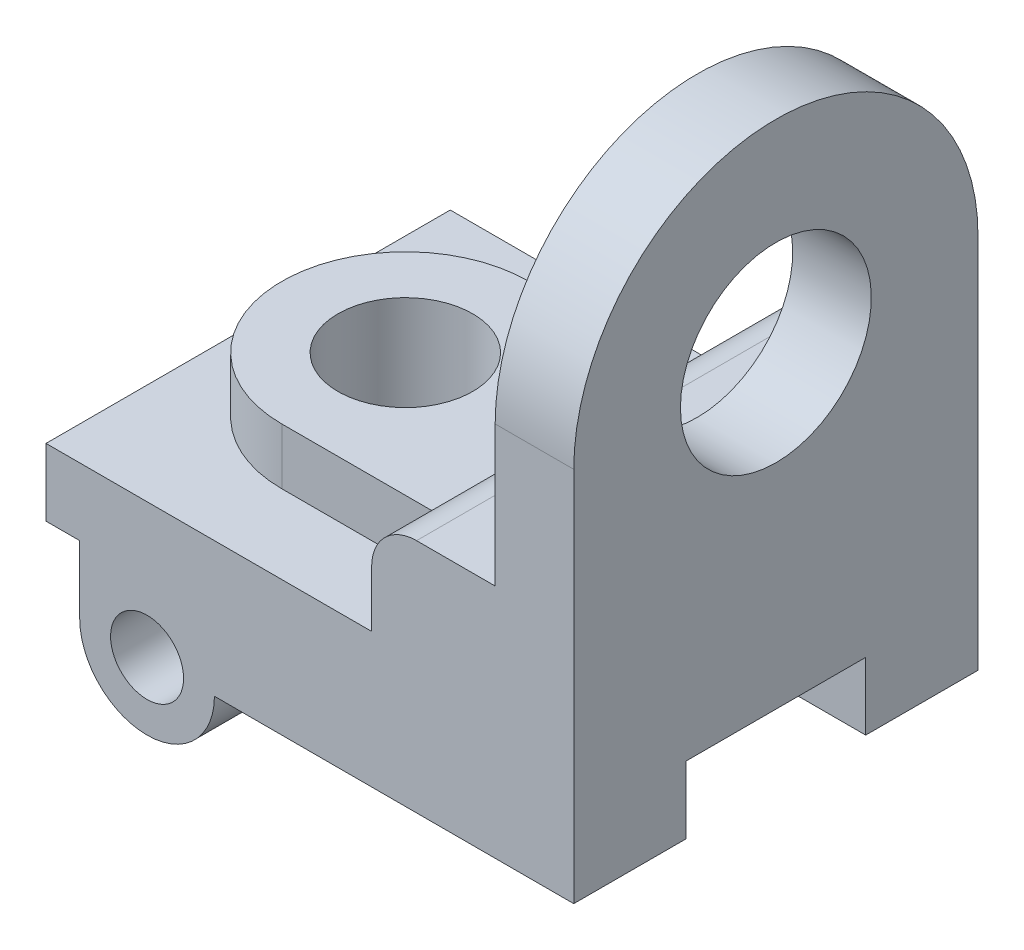
ISO-10303-21;
HEADER;
FILE_DESCRIPTION(('STEP AP214'),'2;1');
FILE_NAME('part.step','',(''),(''),'','','');
FILE_SCHEMA(('AUTOMOTIVE_DESIGN { 1 0 10303 214 1 1 1 1 }'));
ENDSEC;
DATA;
#1=APPLICATION_CONTEXT('core data for automotive mechanical design processes');
#2=APPLICATION_PROTOCOL_DEFINITION('international standard','automotive_design',2000,#1);
#3=PRODUCT_CONTEXT('',#1,'mechanical');
#4=PRODUCT('Part','Part','',(#3));
#5=PRODUCT_RELATED_PRODUCT_CATEGORY('part','',(#4));
#6=PRODUCT_DEFINITION_FORMATION('','',#4);
#7=PRODUCT_DEFINITION_CONTEXT('part definition',#1,'design');
#8=PRODUCT_DEFINITION('design','',#6,#7);
#9=PRODUCT_DEFINITION_SHAPE('','',#8);
#10=(LENGTH_UNIT() NAMED_UNIT(*) SI_UNIT(.MILLI.,.METRE.));
#11=(NAMED_UNIT(*) PLANE_ANGLE_UNIT() SI_UNIT($,.RADIAN.));
#12=(NAMED_UNIT(*) SI_UNIT($,.STERADIAN.) SOLID_ANGLE_UNIT());
#13=UNCERTAINTY_MEASURE_WITH_UNIT(LENGTH_MEASURE(1.E-05),#10,'distance_accuracy_value','');
#14=(GEOMETRIC_REPRESENTATION_CONTEXT(3) GLOBAL_UNCERTAINTY_ASSIGNED_CONTEXT((#13)) GLOBAL_UNIT_ASSIGNED_CONTEXT((#10,
#11,#12)) REPRESENTATION_CONTEXT('',''));
#15=CARTESIAN_POINT('',(0.,0.,0.));
#16=DIRECTION('',(0.,0.,1.));
#17=DIRECTION('',(1.,0.,0.));
#18=AXIS2_PLACEMENT_3D('',#15,#16,#17);
#19=CARTESIAN_POINT('',(-36.,0.,36.));
#20=DIRECTION('',(1.,0.,0.));
#21=DIRECTION('',(0.,0.,-1.));
#22=AXIS2_PLACEMENT_3D('',#19,#20,#21);
#23=PLANE('',#22);
#24=DIRECTION('',(0.,-1.,0.));
#25=VECTOR('',#24,1.);
#26=CARTESIAN_POINT('',(-36.,22.,22.));
#27=LINE('',#26,#25);
#28=CARTESIAN_POINT('',(-36.,22.,22.));
#29=VERTEX_POINT('',#28);
#30=CARTESIAN_POINT('',(-36.,12.,22.));
#31=VERTEX_POINT('',#30);
#32=EDGE_CURVE('E198',#29,#31,#27,.T.);
#33=ORIENTED_EDGE('',*,*,#32,.T.);
#34=DIRECTION('',(0.,0.,-1.));
#35=VECTOR('',#34,1.);
#36=CARTESIAN_POINT('',(-36.,12.,36.));
#37=LINE('',#36,#35);
#38=CARTESIAN_POINT('',(-36.,12.,36.));
#39=VERTEX_POINT('',#38);
#40=EDGE_CURVE('E329',#39,#31,#37,.T.);
#41=ORIENTED_EDGE('',*,*,#40,.F.);
#42=DIRECTION('',(0.,-1.,0.));
#43=VECTOR('',#42,1.);
#44=CARTESIAN_POINT('',(-36.,0.,36.));
#45=LINE('',#44,#43);
#46=CARTESIAN_POINT('',(-36.,22.,36.));
#47=VERTEX_POINT('',#46);
#48=EDGE_CURVE('E276',#47,#39,#45,.T.);
#49=ORIENTED_EDGE('',*,*,#48,.F.);
#50=DIRECTION('',(0.,0.,-1.));
#51=VECTOR('',#50,1.);
#52=CARTESIAN_POINT('',(-36.,22.,36.));
#53=LINE('',#52,#51);
#54=EDGE_CURVE('E331',#47,#29,#53,.T.);
#55=ORIENTED_EDGE('',*,*,#54,.T.);
#56=EDGE_LOOP('',(#33,#41,#49,#55));
#57=FACE_BOUND('',#56,.T.);
#58=ADVANCED_FACE('F41',(#57),#23,.F.);
#59=DIRECTION('',(0.,-1.,0.));
#60=VECTOR('',#59,1.);
#61=CARTESIAN_POINT('',(-36.,22.,-22.));
#62=LINE('',#61,#60);
#63=CARTESIAN_POINT('',(-36.,22.,-22.));
#64=VERTEX_POINT('',#63);
#65=CARTESIAN_POINT('',(-36.,12.,-22.));
#66=VERTEX_POINT('',#65);
#67=EDGE_CURVE('E59',#64,#66,#62,.T.);
#68=ORIENTED_EDGE('',*,*,#67,.F.);
#69=CARTESIAN_POINT('',(-36.,22.,-36.));
#70=VERTEX_POINT('',#69);
#71=EDGE_CURVE('E334',#64,#70,#53,.T.);
#72=ORIENTED_EDGE('',*,*,#71,.T.);
#73=DIRECTION('',(0.,-1.,0.));
#74=VECTOR('',#73,1.);
#75=CARTESIAN_POINT('',(-36.,0.,-36.));
#76=LINE('',#75,#74);
#77=CARTESIAN_POINT('',(-36.,12.,-36.));
#78=VERTEX_POINT('',#77);
#79=EDGE_CURVE('E313',#70,#78,#76,.T.);
#80=ORIENTED_EDGE('',*,*,#79,.T.);
#81=EDGE_CURVE('E328',#66,#78,#37,.T.);
#82=ORIENTED_EDGE('',*,*,#81,.F.);
#83=EDGE_LOOP('',(#68,#72,#80,#82));
#84=FACE_BOUND('',#83,.T.);
#85=ADVANCED_FACE('F436',(#84),#23,.F.);
#86=CARTESIAN_POINT('',(0.,12.,36.));
#87=DIRECTION('',(0.,-1.,0.));
#88=DIRECTION('',(1.,0.,0.));
#89=AXIS2_PLACEMENT_3D('',#86,#87,#88);
#90=PLANE('',#89);
#91=DIRECTION('',(1.,0.,0.));
#92=VECTOR('',#91,1.);
#93=CARTESIAN_POINT('',(-66.,12.,22.));
#94=LINE('',#93,#92);
#95=CARTESIAN_POINT('',(-66.,12.,22.));
#96=VERTEX_POINT('',#95);
#97=EDGE_CURVE('E448',#96,#31,#94,.T.);
#98=ORIENTED_EDGE('',*,*,#97,.F.);
#99=CARTESIAN_POINT('',(-66.,12.,0.));
#100=DIRECTION('',(0.,1.,0.));
#101=DIRECTION('',(-1.,0.,0.));
#102=AXIS2_PLACEMENT_3D('',#99,#100,#101);
#103=CIRCLE('',#102,22.);
#104=CARTESIAN_POINT('',(-66.,12.,-22.));
#105=VERTEX_POINT('',#104);
#106=EDGE_CURVE('E209',#105,#96,#103,.T.);
#107=ORIENTED_EDGE('',*,*,#106,.F.);
#108=DIRECTION('',(-1.,0.,0.));
#109=VECTOR('',#108,1.);
#110=CARTESIAN_POINT('',(-66.,12.,-22.));
#111=LINE('',#110,#109);
#112=EDGE_CURVE('E210',#66,#105,#111,.T.);
#113=ORIENTED_EDGE('',*,*,#112,.F.);
#114=ORIENTED_EDGE('',*,*,#81,.T.);
#115=DIRECTION('',(-1.,0.,0.));
#116=VECTOR('',#115,1.);
#117=CARTESIAN_POINT('',(0.,12.,-36.));
#118=LINE('',#117,#116);
#119=CARTESIAN_POINT('',(-94.,12.,-36.));
#120=VERTEX_POINT('',#119);
#121=EDGE_CURVE('E314',#78,#120,#118,.T.);
#122=ORIENTED_EDGE('',*,*,#121,.T.);
#123=DIRECTION('',(0.,0.,-1.));
#124=VECTOR('',#123,1.);
#125=CARTESIAN_POINT('',(-94.,12.,36.));
#126=LINE('',#125,#124);
#127=CARTESIAN_POINT('',(-94.,12.,36.));
#128=VERTEX_POINT('',#127);
#129=EDGE_CURVE('E326',#128,#120,#126,.T.);
#130=ORIENTED_EDGE('',*,*,#129,.F.);
#131=DIRECTION('',(-1.,0.,0.));
#132=VECTOR('',#131,1.);
#133=CARTESIAN_POINT('',(0.,12.,36.));
#134=LINE('',#133,#132);
#135=EDGE_CURVE('E283',#39,#128,#134,.T.);
#136=ORIENTED_EDGE('',*,*,#135,.F.);
#137=ORIENTED_EDGE('',*,*,#40,.T.);
#138=EDGE_LOOP('',(#98,#107,#113,#114,#122,#130,#136,#137));
#139=FACE_BOUND('',#138,.T.);
#140=ADVANCED_FACE('F418',(#139),#90,.F.);
#141=CARTESIAN_POINT('',(-88.,0.,36.));
#142=DIRECTION('',(1.,0.,0.));
#143=DIRECTION('',(0.,0.,-1.));
#144=AXIS2_PLACEMENT_3D('',#141,#142,#143);
#145=PLANE('',#144);
#146=DIRECTION('',(0.,0.,-1.));
#147=VECTOR('',#146,1.);
#148=CARTESIAN_POINT('',(-88.,-12.,36.));
#149=LINE('',#148,#147);
#150=CARTESIAN_POINT('',(-88.,-12.,-16.));
#151=VERTEX_POINT('',#150);
#152=CARTESIAN_POINT('',(-88.,-12.,-36.));
#153=VERTEX_POINT('',#152);
#154=EDGE_CURVE('E49',#151,#153,#149,.T.);
#155=ORIENTED_EDGE('',*,*,#154,.F.);
#156=DIRECTION('',(0.,-1.,0.));
#157=VECTOR('',#156,1.);
#158=CARTESIAN_POINT('',(-88.,0.,-16.));
#159=LINE('',#158,#157);
#160=CARTESIAN_POINT('',(-88.,0.,-16.));
#161=VERTEX_POINT('',#160);
#162=EDGE_CURVE('E223',#161,#151,#159,.T.);
#163=ORIENTED_EDGE('',*,*,#162,.F.);
#164=DIRECTION('',(0.,0.,-1.));
#165=VECTOR('',#164,1.);
#166=CARTESIAN_POINT('',(-88.,0.,36.));
#167=LINE('',#166,#165);
#168=CARTESIAN_POINT('',(-88.,0.,-36.));
#169=VERTEX_POINT('',#168);
#170=EDGE_CURVE('E290',#161,#169,#167,.T.);
#171=ORIENTED_EDGE('',*,*,#170,.T.);
#172=DIRECTION('',(0.,-1.,0.));
#173=VECTOR('',#172,1.);
#174=CARTESIAN_POINT('',(-88.,0.,-36.));
#175=LINE('',#174,#173);
#176=EDGE_CURVE('E289',#169,#153,#175,.T.);
#177=ORIENTED_EDGE('',*,*,#176,.T.);
#178=EDGE_LOOP('',(#155,#163,#171,#177));
#179=FACE_BOUND('',#178,.T.);
#180=ADVANCED_FACE('F435',(#179),#145,.F.);
#181=CARTESIAN_POINT('',(-76.,-12.,36.));
#182=DIRECTION('',(0.,0.,-1.));
#183=DIRECTION('',(-1.,0.,0.));
#184=AXIS2_PLACEMENT_3D('',#181,#182,#183);
#185=CYLINDRICAL_SURFACE('',#184,12.);
#186=DIRECTION('',(0.,0.,-1.));
#187=VECTOR('',#186,1.);
#188=CARTESIAN_POINT('',(-64.,-12.,36.));
#189=LINE('',#188,#187);
#190=CARTESIAN_POINT('',(-64.,-12.,-16.));
#191=VERTEX_POINT('',#190);
#192=CARTESIAN_POINT('',(-64.,-12.,-36.));
#193=VERTEX_POINT('',#192);
#194=EDGE_CURVE('E347',#191,#193,#189,.T.);
#195=ORIENTED_EDGE('',*,*,#194,.F.);
#196=CARTESIAN_POINT('',(-76.,-12.,-16.));
#197=DIRECTION('',(0.,0.,-1.));
#198=DIRECTION('',(-1.,0.,0.));
#199=AXIS2_PLACEMENT_3D('',#196,#197,#198);
#200=CIRCLE('',#199,12.);
#201=EDGE_CURVE('E254',#191,#151,#200,.T.);
#202=ORIENTED_EDGE('',*,*,#201,.T.);
#203=ORIENTED_EDGE('',*,*,#154,.T.);
#204=CARTESIAN_POINT('',(-76.,-12.,-36.));
#205=DIRECTION('',(0.,0.,1.));
#206=DIRECTION('',(1.,0.,0.));
#207=AXIS2_PLACEMENT_3D('',#204,#205,#206);
#208=CIRCLE('',#207,12.);
#209=EDGE_CURVE('E291',#153,#193,#208,.T.);
#210=ORIENTED_EDGE('',*,*,#209,.T.);
#211=EDGE_LOOP('',(#195,#202,#203,#210));
#212=FACE_BOUND('',#211,.T.);
#213=ADVANCED_FACE('F495',(#212),#185,.T.);
#214=CARTESIAN_POINT('',(0.,-12.,36.));
#215=DIRECTION('',(0.,1.,0.));
#216=DIRECTION('',(0.,0.,1.));
#217=AXIS2_PLACEMENT_3D('',#214,#215,#216);
#218=PLANE('',#217);
#219=DIRECTION('',(0.,0.,-1.));
#220=VECTOR('',#219,1.);
#221=CARTESIAN_POINT('',(0.,-12.,36.));
#222=LINE('',#221,#220);
#223=CARTESIAN_POINT('',(0.,-12.,-16.));
#224=VERTEX_POINT('',#223);
#225=CARTESIAN_POINT('',(0.,-12.,-36.));
#226=VERTEX_POINT('',#225);
#227=EDGE_CURVE('E345',#224,#226,#222,.T.);
#228=ORIENTED_EDGE('',*,*,#227,.F.);
#229=DIRECTION('',(-1.,0.,0.));
#230=VECTOR('',#229,1.);
#231=CARTESIAN_POINT('',(0.,-12.,-16.));
#232=LINE('',#231,#230);
#233=EDGE_CURVE('E252',#224,#191,#232,.T.);
#234=ORIENTED_EDGE('',*,*,#233,.T.);
#235=ORIENTED_EDGE('',*,*,#194,.T.);
#236=DIRECTION('',(1.,0.,0.));
#237=VECTOR('',#236,1.);
#238=CARTESIAN_POINT('',(0.,-12.,-36.));
#239=LINE('',#238,#237);
#240=EDGE_CURVE('E298',#193,#226,#239,.T.);
#241=ORIENTED_EDGE('',*,*,#240,.T.);
#242=EDGE_LOOP('',(#228,#234,#235,#241));
#243=FACE_BOUND('',#242,.T.);
#244=ADVANCED_FACE('F426',(#243),#218,.F.);
#245=CARTESIAN_POINT('',(-76.,-12.,36.));
#246=DIRECTION('',(0.,0.,-1.));
#247=DIRECTION('',(-1.,0.,0.));
#248=AXIS2_PLACEMENT_3D('',#245,#246,#247);
#249=CYLINDRICAL_SURFACE('',#248,6.5);
#250=CARTESIAN_POINT('',(-76.,-12.,-16.));
#251=DIRECTION('',(0.,0.,-1.));
#252=DIRECTION('',(-1.,0.,0.));
#253=AXIS2_PLACEMENT_3D('',#250,#251,#252);
#254=CIRCLE('',#253,6.5);
#255=CARTESIAN_POINT('',(-82.5,-12.,-16.));
#256=VERTEX_POINT('',#255);
#257=EDGE_CURVE('E44',#256,#256,#254,.T.);
#258=ORIENTED_EDGE('',*,*,#257,.F.);
#259=EDGE_LOOP('',(#258));
#260=FACE_BOUND('',#259,.T.);
#261=CARTESIAN_POINT('',(-76.,-12.,-36.));
#262=DIRECTION('',(0.,0.,1.));
#263=DIRECTION('',(1.,0.,0.));
#264=AXIS2_PLACEMENT_3D('',#261,#262,#263);
#265=CIRCLE('',#264,6.5);
#266=CARTESIAN_POINT('',(-69.5,-12.,-36.));
#267=VERTEX_POINT('',#266);
#268=EDGE_CURVE('E260',#267,#267,#265,.T.);
#269=ORIENTED_EDGE('',*,*,#268,.F.);
#270=EDGE_LOOP('',(#269));
#271=FACE_BOUND('',#270,.T.);
#272=ADVANCED_FACE('F357',(#260,#271),#249,.F.);
#273=CARTESIAN_POINT('',(-88.,0.,36.));
#274=VERTEX_POINT('',#273);
#275=CARTESIAN_POINT('',(-88.,0.,16.));
#276=VERTEX_POINT('',#275);
#277=EDGE_CURVE('E319',#274,#276,#167,.T.);
#278=ORIENTED_EDGE('',*,*,#277,.T.);
#279=DIRECTION('',(0.,1.,0.));
#280=VECTOR('',#279,1.);
#281=CARTESIAN_POINT('',(-88.,0.,16.));
#282=LINE('',#281,#280);
#283=CARTESIAN_POINT('',(-88.,-12.,16.));
#284=VERTEX_POINT('',#283);
#285=EDGE_CURVE('E235',#284,#276,#282,.T.);
#286=ORIENTED_EDGE('',*,*,#285,.F.);
#287=CARTESIAN_POINT('',(-88.,-12.,36.));
#288=VERTEX_POINT('',#287);
#289=EDGE_CURVE('E11',#288,#284,#149,.T.);
#290=ORIENTED_EDGE('',*,*,#289,.F.);
#291=DIRECTION('',(0.,-1.,0.));
#292=VECTOR('',#291,1.);
#293=CARTESIAN_POINT('',(-88.,0.,36.));
#294=LINE('',#293,#292);
#295=EDGE_CURVE('E261',#274,#288,#294,.T.);
#296=ORIENTED_EDGE('',*,*,#295,.F.);
#297=EDGE_LOOP('',(#278,#286,#290,#296));
#298=FACE_BOUND('',#297,.T.);
#299=ADVANCED_FACE('F372',(#298),#145,.F.);
#300=CARTESIAN_POINT('',(-76.,-12.,16.));
#301=DIRECTION('',(0.,0.,1.));
#302=DIRECTION('',(0.,-1.,0.));
#303=AXIS2_PLACEMENT_3D('',#300,#301,#302);
#304=CIRCLE('',#303,12.);
#305=CARTESIAN_POINT('',(-64.,-12.,16.));
#306=VERTEX_POINT('',#305);
#307=EDGE_CURVE('E249',#284,#306,#304,.T.);
#308=ORIENTED_EDGE('',*,*,#307,.T.);
#309=CARTESIAN_POINT('',(-64.,-12.,36.));
#310=VERTEX_POINT('',#309);
#311=EDGE_CURVE('E350',#310,#306,#189,.T.);
#312=ORIENTED_EDGE('',*,*,#311,.F.);
#313=CARTESIAN_POINT('',(-76.,-12.,36.));
#314=DIRECTION('',(0.,0.,1.));
#315=DIRECTION('',(1.,0.,0.));
#316=AXIS2_PLACEMENT_3D('',#313,#314,#315);
#317=CIRCLE('',#316,12.);
#318=EDGE_CURVE('E264',#288,#310,#317,.T.);
#319=ORIENTED_EDGE('',*,*,#318,.F.);
#320=ORIENTED_EDGE('',*,*,#289,.T.);
#321=EDGE_LOOP('',(#308,#312,#319,#320));
#322=FACE_BOUND('',#321,.T.);
#323=ADVANCED_FACE('F376',(#322),#185,.T.);
#324=ORIENTED_EDGE('',*,*,#311,.T.);
#325=DIRECTION('',(1.,0.,0.));
#326=VECTOR('',#325,1.);
#327=CARTESIAN_POINT('',(0.,-12.,16.));
#328=LINE('',#327,#326);
#329=CARTESIAN_POINT('',(0.,-12.,16.));
#330=VERTEX_POINT('',#329);
#331=EDGE_CURVE('E250',#306,#330,#328,.T.);
#332=ORIENTED_EDGE('',*,*,#331,.T.);
#333=CARTESIAN_POINT('',(0.,-12.,36.));
#334=VERTEX_POINT('',#333);
#335=EDGE_CURVE('E343',#334,#330,#222,.T.);
#336=ORIENTED_EDGE('',*,*,#335,.F.);
#337=DIRECTION('',(1.,0.,0.));
#338=VECTOR('',#337,1.);
#339=CARTESIAN_POINT('',(0.,-12.,36.));
#340=LINE('',#339,#338);
#341=EDGE_CURVE('E270',#310,#334,#340,.T.);
#342=ORIENTED_EDGE('',*,*,#341,.F.);
#343=EDGE_LOOP('',(#324,#332,#336,#342));
#344=FACE_BOUND('',#343,.T.);
#345=ADVANCED_FACE('F381',(#344),#218,.F.);
#346=CARTESIAN_POINT('',(0.,0.,36.));
#347=DIRECTION('',(-1.,0.,0.));
#348=DIRECTION('',(0.,0.,1.));
#349=AXIS2_PLACEMENT_3D('',#346,#347,#348);
#350=PLANE('',#349);
#351=CARTESIAN_POINT('',(0.,55.,0.));
#352=DIRECTION('',(-1.,0.,0.));
#353=DIRECTION('',(0.,0.,1.));
#354=AXIS2_PLACEMENT_3D('',#351,#352,#353);
#355=CIRCLE('',#354,17.);
#356=CARTESIAN_POINT('',(0.,55.,17.));
#357=VERTEX_POINT('',#356);
#358=EDGE_CURVE('E212',#357,#357,#355,.F.);
#359=ORIENTED_EDGE('',*,*,#358,.F.);
#360=EDGE_LOOP('',(#359));
#361=FACE_BOUND('',#360,.T.);
#362=DIRECTION('',(0.,0.,-1.));
#363=VECTOR('',#362,1.);
#364=CARTESIAN_POINT('',(0.,0.,-16.));
#365=LINE('',#364,#363);
#366=CARTESIAN_POINT('',(0.,0.,16.));
#367=VERTEX_POINT('',#366);
#368=CARTESIAN_POINT('',(0.,0.,-16.));
#369=VERTEX_POINT('',#368);
#370=EDGE_CURVE('E234',#367,#369,#365,.T.);
#371=ORIENTED_EDGE('',*,*,#370,.T.);
#372=DIRECTION('',(0.,-1.,0.));
#373=VECTOR('',#372,1.);
#374=CARTESIAN_POINT('',(0.,0.,-16.));
#375=LINE('',#374,#373);
#376=EDGE_CURVE('E227',#369,#224,#375,.T.);
#377=ORIENTED_EDGE('',*,*,#376,.T.);
#378=ORIENTED_EDGE('',*,*,#227,.T.);
#379=DIRECTION('',(0.,1.,0.));
#380=VECTOR('',#379,1.);
#381=CARTESIAN_POINT('',(0.,0.,-36.));
#382=LINE('',#381,#380);
#383=CARTESIAN_POINT('',(0.,55.,-36.));
#384=VERTEX_POINT('',#383);
#385=EDGE_CURVE('E300',#226,#384,#382,.T.);
#386=ORIENTED_EDGE('',*,*,#385,.T.);
#387=CARTESIAN_POINT('',(0.,55.,0.));
#388=DIRECTION('',(1.,0.,0.));
#389=DIRECTION('',(0.,0.,-1.));
#390=AXIS2_PLACEMENT_3D('',#387,#388,#389);
#391=CIRCLE('',#390,36.);
#392=CARTESIAN_POINT('',(0.,55.,36.));
#393=VERTEX_POINT('',#392);
#394=EDGE_CURVE('E222',#384,#393,#391,.T.);
#395=ORIENTED_EDGE('',*,*,#394,.T.);
#396=DIRECTION('',(0.,1.,0.));
#397=VECTOR('',#396,1.);
#398=CARTESIAN_POINT('',(0.,0.,36.));
#399=LINE('',#398,#397);
#400=EDGE_CURVE('E267',#334,#393,#399,.T.);
#401=ORIENTED_EDGE('',*,*,#400,.F.);
#402=ORIENTED_EDGE('',*,*,#335,.T.);
#403=DIRECTION('',(0.,1.,0.));
#404=VECTOR('',#403,1.);
#405=CARTESIAN_POINT('',(0.,0.,16.));
#406=LINE('',#405,#404);
#407=EDGE_CURVE('E231',#330,#367,#406,.T.);
#408=ORIENTED_EDGE('',*,*,#407,.T.);
#409=EDGE_LOOP('',(#371,#377,#378,#386,#395,#401,#402,#408));
#410=FACE_BOUND('',#409,.T.);
#411=ADVANCED_FACE('F388',(#361,#410),#350,.F.);
#412=CARTESIAN_POINT('',(-14.,0.,36.));
#413=DIRECTION('',(1.,0.,0.));
#414=DIRECTION('',(0.,1.,0.));
#415=AXIS2_PLACEMENT_3D('',#412,#413,#414);
#416=PLANE('',#415);
#417=CARTESIAN_POINT('',(-14.,55.,0.));
#418=DIRECTION('',(-1.,0.,0.));
#419=DIRECTION('',(0.,-1.,0.));
#420=AXIS2_PLACEMENT_3D('',#417,#418,#419);
#421=CIRCLE('',#420,17.);
#422=CARTESIAN_POINT('',(-14.,38.,0.));
#423=VERTEX_POINT('',#422);
#424=EDGE_CURVE('E211',#423,#423,#421,.T.);
#425=ORIENTED_EDGE('',*,*,#424,.F.);
#426=EDGE_LOOP('',(#425));
#427=FACE_BOUND('',#426,.T.);
#428=DIRECTION('',(0.,-1.,0.));
#429=VECTOR('',#428,1.);
#430=CARTESIAN_POINT('',(-14.,0.,-36.));
#431=LINE('',#430,#429);
#432=CARTESIAN_POINT('',(-14.,55.,-36.));
#433=VERTEX_POINT('',#432);
#434=CARTESIAN_POINT('',(-14.,30.,-36.));
#435=VERTEX_POINT('',#434);
#436=EDGE_CURVE('E302',#433,#435,#431,.T.);
#437=ORIENTED_EDGE('',*,*,#436,.T.);
#438=DIRECTION('',(0.,0.,-1.));
#439=VECTOR('',#438,1.);
#440=CARTESIAN_POINT('',(-14.,30.,36.));
#441=LINE('',#440,#439);
#442=CARTESIAN_POINT('',(-14.,30.,36.));
#443=VERTEX_POINT('',#442);
#444=EDGE_CURVE('E340',#443,#435,#441,.T.);
#445=ORIENTED_EDGE('',*,*,#444,.F.);
#446=DIRECTION('',(0.,-1.,0.));
#447=VECTOR('',#446,1.);
#448=CARTESIAN_POINT('',(-14.,0.,36.));
#449=LINE('',#448,#447);
#450=CARTESIAN_POINT('',(-14.,55.,36.));
#451=VERTEX_POINT('',#450);
#452=EDGE_CURVE('E272',#451,#443,#449,.T.);
#453=ORIENTED_EDGE('',*,*,#452,.F.);
#454=CARTESIAN_POINT('',(-14.,55.,0.));
#455=DIRECTION('',(1.,0.,0.));
#456=DIRECTION('',(0.,1.,0.));
#457=AXIS2_PLACEMENT_3D('',#454,#455,#456);
#458=CIRCLE('',#457,36.);
#459=EDGE_CURVE('E225',#451,#433,#458,.F.);
#460=ORIENTED_EDGE('',*,*,#459,.T.);
#461=EDGE_LOOP('',(#437,#445,#453,#460));
#462=FACE_BOUND('',#461,.T.);
#463=ADVANCED_FACE('F402',(#427,#462),#416,.F.);
#464=CARTESIAN_POINT('',(0.,30.,36.));
#465=DIRECTION('',(0.,-1.,0.));
#466=DIRECTION('',(1.,0.,0.));
#467=AXIS2_PLACEMENT_3D('',#464,#465,#466);
#468=PLANE('',#467);
#469=DIRECTION('',(-1.,0.,0.));
#470=VECTOR('',#469,1.);
#471=CARTESIAN_POINT('',(0.,30.,-36.));
#472=LINE('',#471,#470);
#473=CARTESIAN_POINT('',(-28.,30.,-36.));
#474=VERTEX_POINT('',#473);
#475=EDGE_CURVE('E308',#435,#474,#472,.T.);
#476=ORIENTED_EDGE('',*,*,#475,.T.);
#477=DIRECTION('',(0.,0.,-1.));
#478=VECTOR('',#477,1.);
#479=CARTESIAN_POINT('',(-28.,30.,36.));
#480=LINE('',#479,#478);
#481=CARTESIAN_POINT('',(-28.,30.,36.));
#482=VERTEX_POINT('',#481);
#483=EDGE_CURVE('E338',#482,#474,#480,.T.);
#484=ORIENTED_EDGE('',*,*,#483,.F.);
#485=DIRECTION('',(-1.,0.,0.));
#486=VECTOR('',#485,1.);
#487=CARTESIAN_POINT('',(0.,30.,36.));
#488=LINE('',#487,#486);
#489=EDGE_CURVE('E274',#443,#482,#488,.T.);
#490=ORIENTED_EDGE('',*,*,#489,.F.);
#491=ORIENTED_EDGE('',*,*,#444,.T.);
#492=EDGE_LOOP('',(#476,#484,#490,#491));
#493=FACE_BOUND('',#492,.T.);
#494=ADVANCED_FACE('F408',(#493),#468,.F.);
#495=CARTESIAN_POINT('',(-28.,22.,36.));
#496=DIRECTION('',(0.,0.,-1.));
#497=DIRECTION('',(-1.,0.,0.));
#498=AXIS2_PLACEMENT_3D('',#495,#496,#497);
#499=CYLINDRICAL_SURFACE('',#498,8.);
#500=CARTESIAN_POINT('',(-28.,22.,-36.));
#501=DIRECTION('',(0.,0.,1.));
#502=DIRECTION('',(1.,0.,0.));
#503=AXIS2_PLACEMENT_3D('',#500,#501,#502);
#504=CIRCLE('',#503,8.);
#505=EDGE_CURVE('E306',#474,#70,#504,.T.);
#506=ORIENTED_EDGE('',*,*,#505,.T.);
#507=ORIENTED_EDGE('',*,*,#71,.F.);
#508=DIRECTION('',(0.,0.,-1.));
#509=VECTOR('',#508,1.);
#510=CARTESIAN_POINT('',(-36.,22.,22.));
#511=LINE('',#510,#509);
#512=EDGE_CURVE('E61',#29,#64,#511,.T.);
#513=ORIENTED_EDGE('',*,*,#512,.F.);
#514=ORIENTED_EDGE('',*,*,#54,.F.);
#515=CARTESIAN_POINT('',(-28.,22.,36.));
#516=DIRECTION('',(0.,0.,1.));
#517=DIRECTION('',(1.,0.,0.));
#518=AXIS2_PLACEMENT_3D('',#515,#516,#517);
#519=CIRCLE('',#518,8.);
#520=EDGE_CURVE('E280',#482,#47,#519,.T.);
#521=ORIENTED_EDGE('',*,*,#520,.F.);
#522=ORIENTED_EDGE('',*,*,#483,.T.);
#523=EDGE_LOOP('',(#506,#507,#513,#514,#521,#522));
#524=FACE_BOUND('',#523,.T.);
#525=ADVANCED_FACE('F409',(#524),#499,.T.);
#526=CARTESIAN_POINT('',(-94.,0.,36.));
#527=DIRECTION('',(1.,0.,0.));
#528=DIRECTION('',(0.,0.,-1.));
#529=AXIS2_PLACEMENT_3D('',#526,#527,#528);
#530=PLANE('',#529);
#531=DIRECTION('',(0.,-1.,0.));
#532=VECTOR('',#531,1.);
#533=CARTESIAN_POINT('',(-94.,0.,-36.));
#534=LINE('',#533,#532);
#535=CARTESIAN_POINT('',(-94.,0.,-36.));
#536=VERTEX_POINT('',#535);
#537=EDGE_CURVE('E316',#120,#536,#534,.T.);
#538=ORIENTED_EDGE('',*,*,#537,.T.);
#539=DIRECTION('',(0.,0.,-1.));
#540=VECTOR('',#539,1.);
#541=CARTESIAN_POINT('',(-94.,0.,36.));
#542=LINE('',#541,#540);
#543=CARTESIAN_POINT('',(-94.,0.,36.));
#544=VERTEX_POINT('',#543);
#545=EDGE_CURVE('E323',#544,#536,#542,.T.);
#546=ORIENTED_EDGE('',*,*,#545,.F.);
#547=DIRECTION('',(0.,-1.,0.));
#548=VECTOR('',#547,1.);
#549=CARTESIAN_POINT('',(-94.,0.,36.));
#550=LINE('',#549,#548);
#551=EDGE_CURVE('E282',#128,#544,#550,.T.);
#552=ORIENTED_EDGE('',*,*,#551,.F.);
#553=ORIENTED_EDGE('',*,*,#129,.T.);
#554=EDGE_LOOP('',(#538,#546,#552,#553));
#555=FACE_BOUND('',#554,.T.);
#556=ADVANCED_FACE('F358',(#555),#530,.F.);
#557=CARTESIAN_POINT('',(-76.,-12.,16.));
#558=DIRECTION('',(0.,0.,1.));
#559=DIRECTION('',(0.,-1.,0.));
#560=AXIS2_PLACEMENT_3D('',#557,#558,#559);
#561=CIRCLE('',#560,6.5);
#562=CARTESIAN_POINT('',(-76.,-18.5,16.));
#563=VERTEX_POINT('',#562);
#564=EDGE_CURVE('E241',#563,#563,#561,.T.);
#565=ORIENTED_EDGE('',*,*,#564,.F.);
#566=EDGE_LOOP('',(#565));
#567=FACE_BOUND('',#566,.T.);
#568=CARTESIAN_POINT('',(-76.,-12.,36.));
#569=DIRECTION('',(0.,0.,1.));
#570=DIRECTION('',(1.,0.,0.));
#571=AXIS2_PLACEMENT_3D('',#568,#569,#570);
#572=CIRCLE('',#571,6.5);
#573=CARTESIAN_POINT('',(-69.5,-12.,36.));
#574=VERTEX_POINT('',#573);
#575=EDGE_CURVE('E256',#574,#574,#572,.T.);
#576=ORIENTED_EDGE('',*,*,#575,.T.);
#577=EDGE_LOOP('',(#576));
#578=FACE_BOUND('',#577,.T.);
#579=ADVANCED_FACE('F43',(#567,#578),#249,.F.);
#580=CARTESIAN_POINT('',(0.,0.,36.));
#581=DIRECTION('',(0.,1.,0.));
#582=DIRECTION('',(0.,0.,1.));
#583=AXIS2_PLACEMENT_3D('',#580,#581,#582);
#584=PLANE('',#583);
#585=CARTESIAN_POINT('',(-66.,0.,0.));
#586=DIRECTION('',(0.,1.,0.));
#587=DIRECTION('',(0.,0.,1.));
#588=AXIS2_PLACEMENT_3D('',#585,#586,#587);
#589=CIRCLE('',#588,12.);
#590=CARTESIAN_POINT('',(-66.,0.,12.));
#591=VERTEX_POINT('',#590);
#592=EDGE_CURVE('E449',#591,#591,#589,.T.);
#593=ORIENTED_EDGE('',*,*,#592,.T.);
#594=EDGE_LOOP('',(#593));
#595=FACE_BOUND('',#594,.T.);
#596=DIRECTION('',(1.,0.,0.));
#597=VECTOR('',#596,1.);
#598=CARTESIAN_POINT('',(0.,0.,-36.));
#599=LINE('',#598,#597);
#600=EDGE_CURVE('E265',#536,#169,#599,.T.);
#601=ORIENTED_EDGE('',*,*,#600,.T.);
#602=ORIENTED_EDGE('',*,*,#170,.F.);
#603=DIRECTION('',(-1.,0.,0.));
#604=VECTOR('',#603,1.);
#605=CARTESIAN_POINT('',(0.,0.,-16.));
#606=LINE('',#605,#604);
#607=EDGE_CURVE('E242',#369,#161,#606,.T.);
#608=ORIENTED_EDGE('',*,*,#607,.F.);
#609=ORIENTED_EDGE('',*,*,#370,.F.);
#610=DIRECTION('',(-1.,0.,0.));
#611=VECTOR('',#610,1.);
#612=CARTESIAN_POINT('',(0.,0.,16.));
#613=LINE('',#612,#611);
#614=EDGE_CURVE('E236',#367,#276,#613,.T.);
#615=ORIENTED_EDGE('',*,*,#614,.T.);
#616=ORIENTED_EDGE('',*,*,#277,.F.);
#617=DIRECTION('',(1.,0.,0.));
#618=VECTOR('',#617,1.);
#619=CARTESIAN_POINT('',(0.,0.,36.));
#620=LINE('',#619,#618);
#621=EDGE_CURVE('E281',#544,#274,#620,.T.);
#622=ORIENTED_EDGE('',*,*,#621,.F.);
#623=ORIENTED_EDGE('',*,*,#545,.T.);
#624=EDGE_LOOP('',(#601,#602,#608,#609,#615,#616,#622,#623));
#625=FACE_BOUND('',#624,.T.);
#626=ADVANCED_FACE('F360',(#595,#625),#584,.F.);
#627=CARTESIAN_POINT('',(0.,0.,36.));
#628=DIRECTION('',(0.,0.,1.));
#629=DIRECTION('',(1.,0.,0.));
#630=AXIS2_PLACEMENT_3D('',#627,#628,#629);
#631=PLANE('',#630);
#632=ORIENTED_EDGE('',*,*,#575,.F.);
#633=EDGE_LOOP('',(#632));
#634=FACE_BOUND('',#633,.T.);
#635=ORIENTED_EDGE('',*,*,#295,.T.);
#636=ORIENTED_EDGE('',*,*,#318,.T.);
#637=ORIENTED_EDGE('',*,*,#341,.T.);
#638=ORIENTED_EDGE('',*,*,#400,.T.);
#639=DIRECTION('',(-1.,0.,0.));
#640=VECTOR('',#639,1.);
#641=CARTESIAN_POINT('',(0.,55.,36.));
#642=LINE('',#641,#640);
#643=EDGE_CURVE('E271',#393,#451,#642,.T.);
#644=ORIENTED_EDGE('',*,*,#643,.T.);
#645=ORIENTED_EDGE('',*,*,#452,.T.);
#646=ORIENTED_EDGE('',*,*,#489,.T.);
#647=ORIENTED_EDGE('',*,*,#520,.T.);
#648=ORIENTED_EDGE('',*,*,#48,.T.);
#649=ORIENTED_EDGE('',*,*,#135,.T.);
#650=ORIENTED_EDGE('',*,*,#551,.T.);
#651=ORIENTED_EDGE('',*,*,#621,.T.);
#652=EDGE_LOOP('',(#635,#636,#637,#638,#644,#645,#646,#647,#648,#649,#650,#651));
#653=FACE_BOUND('',#652,.T.);
#654=ADVANCED_FACE('F362',(#634,#653),#631,.T.);
#655=CARTESIAN_POINT('',(0.,0.,-36.));
#656=DIRECTION('',(0.,0.,1.));
#657=DIRECTION('',(1.,0.,0.));
#658=AXIS2_PLACEMENT_3D('',#655,#656,#657);
#659=PLANE('',#658);
#660=ORIENTED_EDGE('',*,*,#268,.T.);
#661=EDGE_LOOP('',(#660));
#662=FACE_BOUND('',#661,.T.);
#663=ORIENTED_EDGE('',*,*,#176,.F.);
#664=ORIENTED_EDGE('',*,*,#600,.F.);
#665=ORIENTED_EDGE('',*,*,#537,.F.);
#666=ORIENTED_EDGE('',*,*,#121,.F.);
#667=ORIENTED_EDGE('',*,*,#79,.F.);
#668=ORIENTED_EDGE('',*,*,#505,.F.);
#669=ORIENTED_EDGE('',*,*,#475,.F.);
#670=ORIENTED_EDGE('',*,*,#436,.F.);
#671=DIRECTION('',(-1.,0.,0.));
#672=VECTOR('',#671,1.);
#673=CARTESIAN_POINT('',(0.,55.,-36.));
#674=LINE('',#673,#672);
#675=EDGE_CURVE('E301',#384,#433,#674,.T.);
#676=ORIENTED_EDGE('',*,*,#675,.F.);
#677=ORIENTED_EDGE('',*,*,#385,.F.);
#678=ORIENTED_EDGE('',*,*,#240,.F.);
#679=ORIENTED_EDGE('',*,*,#209,.F.);
#680=EDGE_LOOP('',(#663,#664,#665,#666,#667,#668,#669,#670,#676,#677,#678,#679));
#681=FACE_BOUND('',#680,.T.);
#682=ADVANCED_FACE('F364',(#662,#681),#659,.F.);
#683=CARTESIAN_POINT('',(0.,0.,-16.));
#684=DIRECTION('',(0.,0.,-1.));
#685=DIRECTION('',(-1.,0.,0.));
#686=AXIS2_PLACEMENT_3D('',#683,#684,#685);
#687=PLANE('',#686);
#688=ORIENTED_EDGE('',*,*,#257,.T.);
#689=EDGE_LOOP('',(#688));
#690=FACE_BOUND('',#689,.T.);
#691=ORIENTED_EDGE('',*,*,#201,.F.);
#692=ORIENTED_EDGE('',*,*,#233,.F.);
#693=ORIENTED_EDGE('',*,*,#376,.F.);
#694=ORIENTED_EDGE('',*,*,#607,.T.);
#695=ORIENTED_EDGE('',*,*,#162,.T.);
#696=EDGE_LOOP('',(#691,#692,#693,#694,#695));
#697=FACE_BOUND('',#696,.T.);
#698=ADVANCED_FACE('F553',(#690,#697),#687,.F.);
#699=CARTESIAN_POINT('',(0.,0.,16.));
#700=DIRECTION('',(0.,0.,1.));
#701=DIRECTION('',(0.,-1.,0.));
#702=AXIS2_PLACEMENT_3D('',#699,#700,#701);
#703=PLANE('',#702);
#704=ORIENTED_EDGE('',*,*,#564,.T.);
#705=EDGE_LOOP('',(#704));
#706=FACE_BOUND('',#705,.T.);
#707=ORIENTED_EDGE('',*,*,#285,.T.);
#708=ORIENTED_EDGE('',*,*,#614,.F.);
#709=ORIENTED_EDGE('',*,*,#407,.F.);
#710=ORIENTED_EDGE('',*,*,#331,.F.);
#711=ORIENTED_EDGE('',*,*,#307,.F.);
#712=EDGE_LOOP('',(#707,#708,#709,#710,#711));
#713=FACE_BOUND('',#712,.T.);
#714=ADVANCED_FACE('F354',(#706,#713),#703,.F.);
#715=CARTESIAN_POINT('',(-94.4984471899924,55.,0.));
#716=DIRECTION('',(1.,0.,0.));
#717=DIRECTION('',(0.,0.,-1.));
#718=AXIS2_PLACEMENT_3D('',#715,#716,#717);
#719=CYLINDRICAL_SURFACE('',#718,36.);
#720=ORIENTED_EDGE('',*,*,#459,.F.);
#721=ORIENTED_EDGE('',*,*,#643,.F.);
#722=ORIENTED_EDGE('',*,*,#394,.F.);
#723=ORIENTED_EDGE('',*,*,#675,.T.);
#724=EDGE_LOOP('',(#720,#721,#722,#723));
#725=FACE_BOUND('',#724,.T.);
#726=ADVANCED_FACE('F386',(#725),#719,.T.);
#727=CARTESIAN_POINT('',(0.0010000000000062,55.,0.));
#728=DIRECTION('',(-1.,0.,0.));
#729=DIRECTION('',(0.,-1.,0.));
#730=AXIS2_PLACEMENT_3D('',#727,#728,#729);
#731=CYLINDRICAL_SURFACE('',#730,17.);
#732=ORIENTED_EDGE('',*,*,#424,.T.);
#733=EDGE_LOOP('',(#732));
#734=FACE_BOUND('',#733,.T.);
#735=ORIENTED_EDGE('',*,*,#358,.T.);
#736=EDGE_LOOP('',(#735));
#737=FACE_BOUND('',#736,.T.);
#738=ADVANCED_FACE('F525',(#734,#737),#731,.F.);
#739=CARTESIAN_POINT('',(-66.,22.,0.));
#740=DIRECTION('',(0.,-1.,0.));
#741=DIRECTION('',(1.,0.,0.));
#742=AXIS2_PLACEMENT_3D('',#739,#740,#741);
#743=CYLINDRICAL_SURFACE('',#742,22.);
#744=ORIENTED_EDGE('',*,*,#106,.T.);
#745=DIRECTION('',(0.,-1.,0.));
#746=VECTOR('',#745,1.);
#747=CARTESIAN_POINT('',(-66.,22.,22.));
#748=LINE('',#747,#746);
#749=CARTESIAN_POINT('',(-66.,22.,22.));
#750=VERTEX_POINT('',#749);
#751=EDGE_CURVE('E192',#750,#96,#748,.T.);
#752=ORIENTED_EDGE('',*,*,#751,.F.);
#753=CARTESIAN_POINT('',(-66.,22.,0.));
#754=DIRECTION('',(0.,1.,0.));
#755=DIRECTION('',(-1.,0.,0.));
#756=AXIS2_PLACEMENT_3D('',#753,#754,#755);
#757=CIRCLE('',#756,22.);
#758=CARTESIAN_POINT('',(-66.,22.,-22.));
#759=VERTEX_POINT('',#758);
#760=EDGE_CURVE('E196',#759,#750,#757,.T.);
#761=ORIENTED_EDGE('',*,*,#760,.F.);
#762=DIRECTION('',(0.,-1.,0.));
#763=VECTOR('',#762,1.);
#764=CARTESIAN_POINT('',(-66.,22.,-22.));
#765=LINE('',#764,#763);
#766=EDGE_CURVE('E442',#759,#105,#765,.T.);
#767=ORIENTED_EDGE('',*,*,#766,.T.);
#768=EDGE_LOOP('',(#744,#752,#761,#767));
#769=FACE_BOUND('',#768,.T.);
#770=ADVANCED_FACE('F207',(#769),#743,.T.);
#771=CARTESIAN_POINT('',(-66.,22.,22.));
#772=DIRECTION('',(0.,0.,-1.));
#773=DIRECTION('',(-1.,0.,0.));
#774=AXIS2_PLACEMENT_3D('',#771,#772,#773);
#775=PLANE('',#774);
#776=ORIENTED_EDGE('',*,*,#97,.T.);
#777=ORIENTED_EDGE('',*,*,#32,.F.);
#778=DIRECTION('',(1.,0.,0.));
#779=VECTOR('',#778,1.);
#780=CARTESIAN_POINT('',(-66.,22.,22.));
#781=LINE('',#780,#779);
#782=EDGE_CURVE('E190',#750,#29,#781,.T.);
#783=ORIENTED_EDGE('',*,*,#782,.F.);
#784=ORIENTED_EDGE('',*,*,#751,.T.);
#785=EDGE_LOOP('',(#776,#777,#783,#784));
#786=FACE_BOUND('',#785,.T.);
#787=ADVANCED_FACE('F195',(#786),#775,.F.);
#788=CARTESIAN_POINT('',(-66.,22.,-22.));
#789=DIRECTION('',(0.,0.,1.));
#790=DIRECTION('',(1.,0.,0.));
#791=AXIS2_PLACEMENT_3D('',#788,#789,#790);
#792=PLANE('',#791);
#793=ORIENTED_EDGE('',*,*,#112,.T.);
#794=ORIENTED_EDGE('',*,*,#766,.F.);
#795=DIRECTION('',(-1.,0.,0.));
#796=VECTOR('',#795,1.);
#797=CARTESIAN_POINT('',(-66.,22.,-22.));
#798=LINE('',#797,#796);
#799=EDGE_CURVE('E201',#64,#759,#798,.T.);
#800=ORIENTED_EDGE('',*,*,#799,.F.);
#801=ORIENTED_EDGE('',*,*,#67,.T.);
#802=EDGE_LOOP('',(#793,#794,#800,#801));
#803=FACE_BOUND('',#802,.T.);
#804=ADVANCED_FACE('F439',(#803),#792,.F.);
#805=CARTESIAN_POINT('',(-66.,22.,0.));
#806=DIRECTION('',(0.,1.,0.));
#807=DIRECTION('',(-1.,0.,0.));
#808=AXIS2_PLACEMENT_3D('',#805,#806,#807);
#809=PLANE('',#808);
#810=CARTESIAN_POINT('',(-66.,22.,0.));
#811=DIRECTION('',(0.,1.,0.));
#812=DIRECTION('',(-1.,0.,0.));
#813=AXIS2_PLACEMENT_3D('',#810,#811,#812);
#814=CIRCLE('',#813,12.);
#815=CARTESIAN_POINT('',(-78.,22.,0.));
#816=VERTEX_POINT('',#815);
#817=EDGE_CURVE('E446',#816,#816,#814,.T.);
#818=ORIENTED_EDGE('',*,*,#817,.F.);
#819=EDGE_LOOP('',(#818));
#820=FACE_BOUND('',#819,.T.);
#821=ORIENTED_EDGE('',*,*,#760,.T.);
#822=ORIENTED_EDGE('',*,*,#782,.T.);
#823=ORIENTED_EDGE('',*,*,#512,.T.);
#824=ORIENTED_EDGE('',*,*,#799,.T.);
#825=EDGE_LOOP('',(#821,#822,#823,#824));
#826=FACE_BOUND('',#825,.T.);
#827=ADVANCED_FACE('F203',(#820,#826),#809,.T.);
#828=CARTESIAN_POINT('',(-66.,-24.,0.));
#829=DIRECTION('',(0.,1.,0.));
#830=DIRECTION('',(-1.,0.,0.));
#831=AXIS2_PLACEMENT_3D('',#828,#829,#830);
#832=CYLINDRICAL_SURFACE('',#831,12.);
#833=ORIENTED_EDGE('',*,*,#817,.T.);
#834=EDGE_LOOP('',(#833));
#835=FACE_BOUND('',#834,.T.);
#836=ORIENTED_EDGE('',*,*,#592,.F.);
#837=EDGE_LOOP('',(#836));
#838=FACE_BOUND('',#837,.T.);
#839=ADVANCED_FACE('F456',(#835,#838),#832,.F.);
#840=CLOSED_SHELL('',(#58,#85,#140,#180,#213,#244,#272,#299,#323,#345,#411,#463,#494,#525,#556,
#579,#626,#654,#682,#698,#714,#726,#738,#770,#787,#804,#827,#839));
#841=MANIFOLD_SOLID_BREP('B2',#840);
#842=ADVANCED_BREP_SHAPE_REPRESENTATION('',(#18,#841),#14);
#843=SHAPE_DEFINITION_REPRESENTATION(#9,#842);
ENDSEC;
END-ISO-10303-21;
